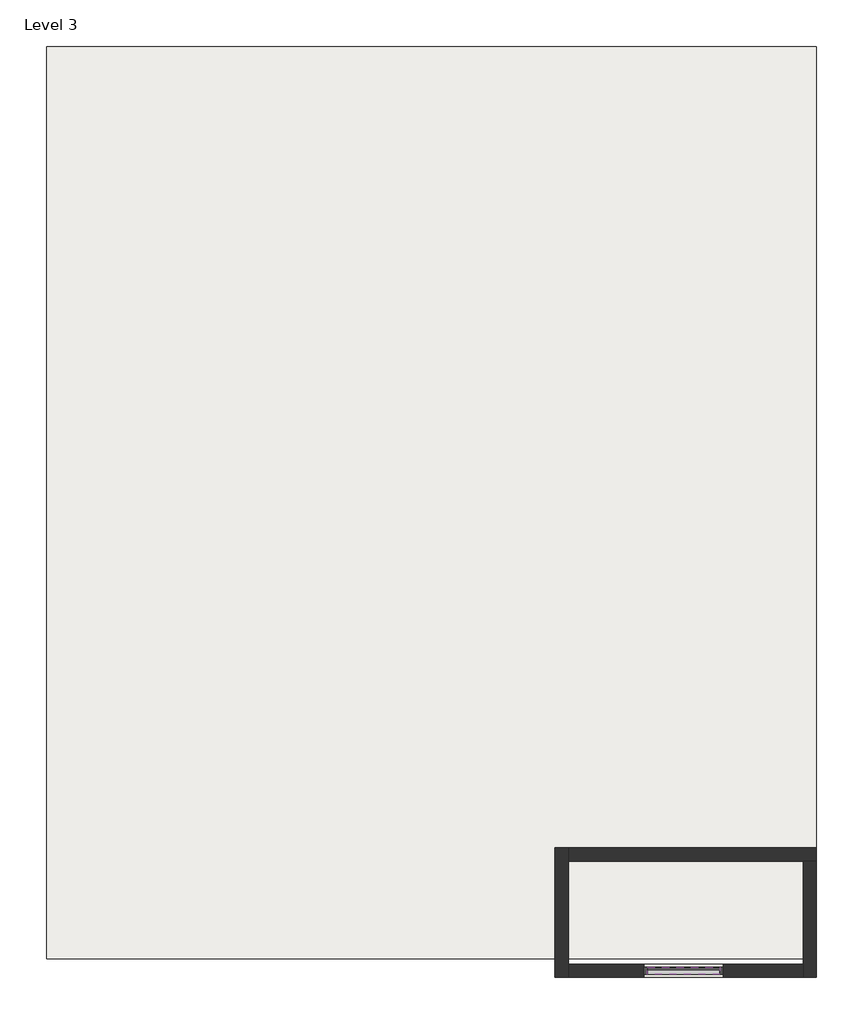
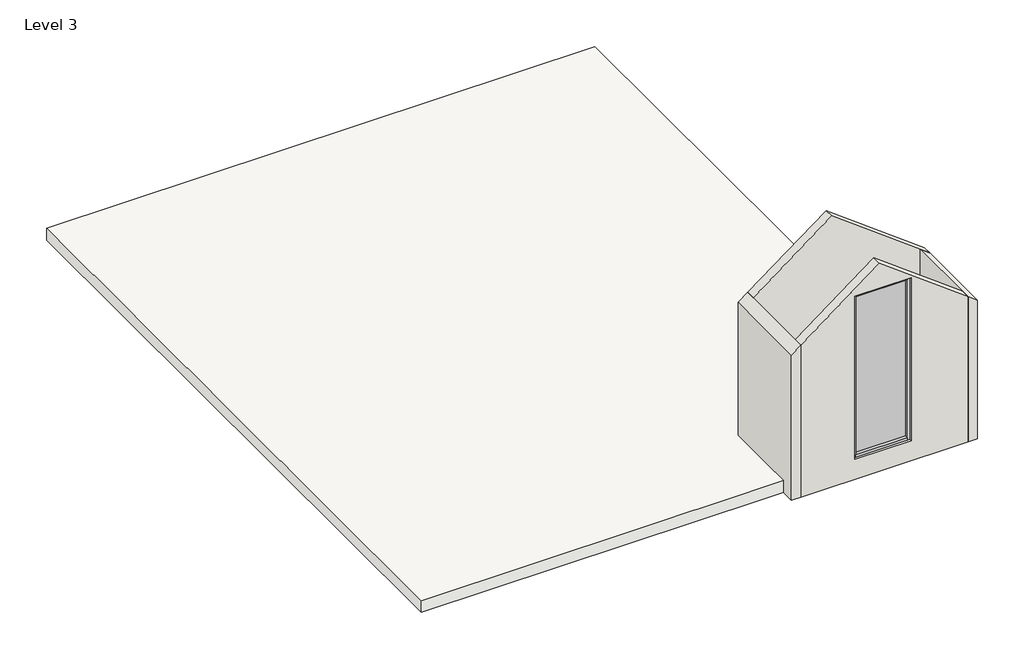
# One storey: 4 members, 4 walls, 1 plate, 1 roof.
"""IFC4 building model written with IfcOpenShell, lengths in millimetres."""

from ifc_helpers import new_model, si_unit, frame, origin, place, context, project, spatial, polyline, outline, extrude, faceted_brep, transform, mapped, element, save
from components import member_73efc3c0, member_71eb4692, system_panel_glazed_716fcd61

model = new_model("IFC4")

# Units and contexts
model_context = context("Model", 3, world=origin())
ifc_project = project(units=[si_unit("LENGTHUNIT", "METRE", prefix="MILLI")], contexts=[model_context])

# Site, building, storey
site = spatial("IfcSite", under=ifc_project)
building = spatial("IfcBuilding", under=site)
storey = spatial("IfcBuildingStorey", under=building, Name="Level 3", Elevation=6096.0)

# Members
placement = place(None, origin())
member_shape = member_73efc3c0(model_context)
element("IfcMember", 1, ObjectType="Rectangular Mullion : 2.5\" x 5\" rectangular", at=placement, inside=storey, context=model_context, shape_type="MappedRepresentation", body=[
    mapped(member_shape, transform((-7141.8761094, -15069.7066876, 6605.1512354), x_axis=(1.0, 0.0, 0.0), y_axis=(0.0, -1.0, 0.0), z_axis=(0.0, 0.0, -1.0))),
])
member_2_shape = member_71eb4692(model_context)
element("IfcMember", 2, ObjectType="Rectangular Mullion : 2.5\" x 5\" rectangular", at=placement, inside=storey, context=model_context, shape_type="MappedRepresentation", body=[
    mapped(member_2_shape, transform((-7205.3761094, -15069.7066876, 10768.2499117), x_axis=(0.0, 0.0, 1.0), y_axis=(0.0, -1.0, 0.0), z_axis=(1.0, 0.0, 0.0))),
])
element("IfcMember", 3, ObjectType="Rectangular Mullion : 2.5\" x 5\" rectangular", at=placement, inside=storey, context=model_context, shape_type="MappedRepresentation", body=[
    mapped(member_2_shape, transform((-8449.9761094, -15069.7066876, 6605.1512354), x_axis=(0.0, 0.0, -1.0), y_axis=(0.0, -1.0, 0.0), z_axis=(-1.0, 0.0, 0.0))),
])
element("IfcMember", 4, ObjectType="Rectangular Mullion : 2.5\" x 5\" rectangular", at=placement, inside=storey, context=model_context, shape_type="MappedRepresentation", body=[
    mapped(member_shape, transform((-8513.4761094, -15069.7066876, 10768.2499117), x_axis=(-1.0, 0.0, 0.0), y_axis=(0.0, -1.0, 0.0), z_axis=(0.0, 0.0, 1.0))),
])

# Plate
system_panel_glazed_shape = system_panel_glazed_716fcd61(model_context)
element("IfcPlate", 5, ObjectType="System Panel : Glazed", at=placement, inside=storey, context=model_context, shape_type="MappedRepresentation", body=[
    mapped(system_panel_glazed_shape, transform((-7827.6761094, -15069.7066876, 6668.6512354), x_axis=(1.0, 0.0, 0.0), y_axis=(0.0, 1.0, 0.0), z_axis=(0.0, 0.0, 1.0))),
])

# Roof
element("IfcRoof", 6, ObjectType="Generic - 12\"", at=placement, inside=storey, context=model_context, shape_type="SweptSolid", body=[
    extrude(outline(polyline([(-18800.4761094, 837.053851), (-5541.6761094, 837.053851), (-5541.6761094, -14860.146149), (-18800.4761094, -14860.146149), (-18800.4761094, 837.053851)])), frame((0.0, 0.0, 6096.0), z_axis=(0.0, 0.0, 1.0), x_axis=(1.0, 0.0, 0.0)), (0.0, 0.0, 1.0), 304.8),
])

# Walls
element("IfcWall", 7, ObjectType="9\"", at=placement, inside=storey, context=model_context, shape_type="Brep", body=[
    faceted_brep([(-9813.0127844, -15184.0066876, 6096.0), (-9813.0127844, -14955.4066876, 6096.0), (-9813.0127844, -13183.746149, 6096.0), (-9813.0127844, -12955.146149, 6096.0), (-9813.0127844, -12955.146149, 9976.7024328), (-9813.0127844, -13183.746149, 9976.7024328), (-9813.0127844, -14955.4066876, 9976.7024328), (-9813.0127844, -15184.0066876, 9976.7024328), (-10041.6127844, -15184.0066876, 6096.0), (-10041.6127844, -15184.0066876, 9805.2524328), (-10041.6127844, -12955.146149, 9805.2524328), (-10041.6127844, -12955.146149, 6096.0)], [[[0, 1, 2, 3, 4, 5, 6, 7]], [[8, 9, 10, 11]], [[3, 2, 1, 0, 8, 11]], [[4, 3, 11, 10]], [[0, 7, 9, 8]], [[7, 6, 5, 4, 10, 9]]]),
])
element("IfcWall", 8, ObjectType="9\"", at=placement, inside=storey, context=model_context, shape_type="Brep", body=[
    faceted_brep([(-9813.0127844, -13183.746149, 6096.0), (-5770.2761094, -13183.746149, 6096.0), (-5541.6761094, -13183.746149, 6096.0), (-5541.6761094, -13183.746149, 9625.5613072), (-5770.2761094, -13183.746149, 9797.0113072), (-7911.4385306, -13183.746149, 11402.8831231), (-9813.0127844, -13183.746149, 9976.7024328), (-9813.0127844, -12955.146149, 6096.0), (-9813.0127844, -12955.146149, 9976.7024328), (-7911.4385306, -12955.146149, 11402.8831231), (-5541.6761094, -12955.146149, 9625.5613072), (-5541.6761094, -12955.146149, 6096.0)], [[[0, 1, 2, 3, 4, 5, 6]], [[7, 8, 9, 10, 11]], [[2, 1, 0, 7, 11]], [[0, 6, 8, 7]], [[3, 2, 11, 10]], [[6, 5, 9, 8]], [[5, 4, 3, 10, 9]]]),
])
element("IfcWall", 9, ObjectType="9\"", at=placement, inside=storey, context=model_context, shape_type="Brep", body=[
    faceted_brep([(-5770.2761094, -13183.746149, 6096.0), (-5770.2761094, -14955.4066876, 6096.0), (-5770.2761094, -15184.0066876, 6096.0), (-5770.2761094, -15184.0066876, 9797.0113072), (-5770.2761094, -14955.4066876, 9797.0113072), (-5770.2761094, -13183.746149, 9797.0113072), (-5541.6761094, -13183.746149, 6096.0), (-5541.6761094, -13183.746149, 9625.5613072), (-5541.6761094, -15184.0066876, 9625.5613072), (-5541.6761094, -15184.0066876, 6096.0)], [[[0, 1, 2, 3, 4, 5]], [[6, 7, 8, 9]], [[2, 1, 0, 6, 9]], [[0, 5, 7, 6]], [[3, 2, 9, 8]], [[5, 4, 3, 8, 7]]]),
])
element("IfcWall", 10, ObjectType="9\"", at=placement, inside=storey, context=model_context, shape_type="SweptSolid", body=[
    extrude(outline(polyline([(6096.0, -9813.0127844), (6096.0, -5770.2761094), (9797.0113072, -5770.2761094), (11402.8831231, -7911.4385306), (9976.7024328, -9813.0127844), (6096.0, -9813.0127844)]), holes=[polyline([(6605.1512354, -8513.4761094), (10768.2499117, -8513.4761094), (10768.2499117, -7141.8761094), (6605.1512354, -7141.8761094), (6605.1512354, -8513.4761094)])]), frame((0.0, -15184.0066876, 0.0), z_axis=(0.0, 1.0, 0.0), x_axis=(0.0, 0.0, 1.0)), (0.0, 0.0, 1.0), 228.6),
])

save(model, "model.ifc")

# Revit data of these elements
# Type "Rectangular Mullion : 2.5\" x 5\" rectangular"
#   built-in parameter 1007304 = 0.416667 (stored number, unit not read)
#   built-in parameter 1007301 = 0.104167 (stored number, unit not read)
#   built-in parameter 1007300 = 0.104167 (stored number, unit not read)
# Type "System Panel : Glazed"
#   Construction Type Id = "GSP4R"
#   Analytic Construction = "1/8 in Pilkington single glazing"
#   Visual Light Transmittance = 0.9
#   Solar Heat Gain Coefficient = 0.86
#   Heat Transfer Coefficient (U) = 1.18115 BTU/(h·ft²·°F)
#   Define Thermal Properties by = 1
# Type "Generic - 12\""
#   Assembly Code = "B1020"
#   Layers, outside or top first: 1' - 0" no material (function 1)
# Type "9\""
#   Assembly Code = "B2010"
#   Layers, outside or top first: 0' - 9" no material (function 1)
# Elements 1, 2, 3, 4 (IfcMember, "Rectangular Mullion : 2.5\" x 5\" rectangular")
#   Phase Created = New Construction
#   Materials on its faces: "Aluminum"
# Element 5 (IfcPlate, "System Panel : Glazed")
#   Phase Created = New Construction
#   Materials on its faces: "Glass"
# Element 6 (IfcRoof, "Generic - 12\"")
#   built-in parameter 1001705 = 21 (stored number, unit not read)
#   built-in parameter 1001710 = 33615
#   Phase Created = New Construction
#   Materials on its faces: "Default Roof"
# Elements 7, 8, 9, 10 (IfcWall, "9\"")
#   Top Offset = 0' - 0"
#   Base Offset = 0' - 0"
#   Unconnected Height = 10' - 0"
#   wall height = 10' - 0"
#   Phase Created = New Construction
#   Base Constraint = Level 3
#   Materials on its faces: "Default Wall"
# Materials
#   "Aluminum": class "Metal", colour RGB 247 247 247, transparency 0, Description = "Aluminum 6061", Cost = 0
#   "Glass": class "Glass", colour RGB 0 128 192, transparency 0.75, Description = "Soda Lime Glass", Cost = 0
#   "Default Roof": colour RGB 88 101 114, transparency 0, Cost = 0
#   "Default Wall": colour RGB 128 128 128, transparency 0, Cost = 0
